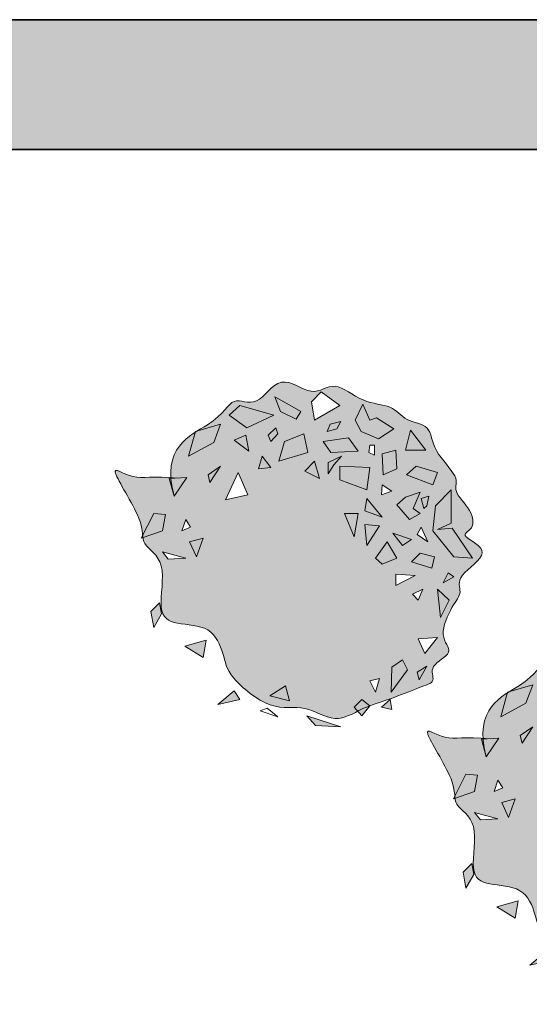
# Model space of a CAD drawing. Units: metres. Extents: x 4298.5 to 4325.2, y 2075 to 2095.8.
# Tile 13 of 35: x 4303.606 to 4304.508, y 2083.045 to 2084.788. Entities that reach past the tile are written whole.
import ezdxf

# ---------------------------------------------------------------- set-up
doc = ezdxf.new("R2010")
doc.units = ezdxf.units.M
for name, color, linetype, lineweight in [('A-ANNO-DIMS', 2, 'Continuous', 18), ('A-WALL', 7, 'Continuous', 35), ('A-WALL-PATT', 252, 'Continuous', 13), ('L-PLNT', 94, 'Continuous', 13)]:
    doc.layers.add(name, color=color, linetype=linetype, lineweight=lineweight)
doc.layers.add('L-PLNT-PATT', color=116, linetype='Continuous', lineweight=13, true_color=0x13823e)
doc.styles.get("Standard").update_dxf_attribs({"font": 'arial.ttf'})
doc.dimstyles.get("Standard").update_dxf_attribs({"dimtxt": 0.18, "dimasz": 0.18, "dimexe": 0.18, "dimexo": 0.0625, "dimgap": 0.09, "dimtad": 0, "dimtih": 1, "dimtoh": 1, "dimdec": 4, "dimzin": 0, "dimdsep": 46, "dimtxsty": 'Standard', "dimcen": 0.09, "dimadec": 0, "dimazin": 0, "dimtfac": 1, "dimtdec": 4, "dimtofl": 0, "dimtmove": 0, "dimatfit": 3, "dimfxl": 1, "dimtolj": 1, "dimtzin": 0, "dimarcsym": 0})

# ---------------------------------------------------------------- blocks, each defined once
blk = doc.blocks.new('*U9')
for points in [[(1.237, 12.003), (0.562, 11.31), (0.764, 10.013), (2.519, 11.051)], [(-4.432, 11.051), (-5.175, 10.359), (-3.96, 9.493), (-2.07, 10.359)], [(-2.003, 11.656), (-1.598, 10.618), (-0.518, 10.099), (-0.181, 10.618), (-0.788, 10.964)], [(4.139, 11.137), (3.599, 10.013), (4.004, 9.234), (5.218, 8.715), (6.298, 9.407), (5.083, 10.186), (4.611, 10.013)], [(-5.782, 9.753), (-7.537, 9.234), (-8.009, 7.504), (-6.255, 8.455)], [(2.586, 9.926), (1.844, 9.753), (1.642, 9.234), (2.316, 9.407)], [(-4.837, 8.628), (-3.825, 7.85), (-4.027, 8.974)], [(-1.935, 9.493), (-2.475, 8.974), (-2.273, 8.542), (-1.8, 9.061)], [(0.022, 9.061), (-1.328, 8.542), (-1.733, 7.157), (0.292, 7.763)], [(7.446, 9.32), (7.108, 7.936), (8.525, 7.936)], [(1.372, 8.542), (3.126, 8.801), (3.801, 7.85), (1.912, 7.763)], [(4.611, 8.282), (4.544, 7.763), (4.949, 7.59), (4.949, 8.282)], [(6.433, 7.936), (5.488, 7.676), (5.556, 6.206), (6.501, 6.638)], [(-2.88, 7.504), (-3.15, 6.638), (-2.273, 6.725)], [(0.764, 7.157), (0.089, 6.465), (1.102, 5.946)], [(1.709, 6.292), (1.709, 7.071), (2.654, 7.504), (2.114, 6.898)], [(-5.782, 6.811), (-6.659, 6.206), (-6.524, 5.687)], [(-4.567, 6.379), (-5.445, 4.475), (-3.892, 4.821)], [(2.519, 6.811), (2.519, 5.86), (4.409, 5.167), (4.611, 6.725)], [(7.851, 6.811), (7.176, 6.206), (8.998, 5.514), (9.335, 6.379)], [(-8.144, 6.033), (-9.359, 5.946), (-9.022, 4.735)], [(5.488, 5.514), (5.421, 4.821), (6.163, 5.081)], [(8.12, 4.994), (7.108, 4.648), (6.501, 4.129), (7.378, 3.091), (8.12, 3.524), (7.648, 3.87)], [(10.28, 5.167), (9.2, 4.043), (8.998, 2.312), (10.482, 0.495), (11.765, 0.409), (10.348, 2.485), (9.335, 2.399), (10.28, 2.831)], [(4.409, 4.562), (4.274, 3.697), (5.488, 3.264)], [(8.728, 4.735), (8.188, 4.562), (8.39, 3.87), (8.593, 4.043)], [(-11.316, 1.793), (-9.831, 2.312), (-9.629, 3.437), (-10.439, 3.524)], [(3.531, 1.88), (2.856, 3.524), (3.801, 3.524)], [(-8.212, 3.091), (-8.482, 2.312), (-7.874, 2.572)], [(4.274, 2.745), (5.286, 2.658), (4.409, 1.274)], [(7.513, 1.707), (6.906, 1.274), (6.231, 2.139)], [(8.188, 2.572), (7.918, 2.053), (8.66, 1.534)], [(-6.997, 1.793), (-7.942, 1.534), (-7.469, 0.495)], [(5.826, 1.534), (5.016, 0.409), (5.488, -0.024), (6.501, 0.409)], [(-8.212, 0.409), (-9.426, 0.322), (-9.831, 0.841)], [(8.12, 0.755), (7.513, 0.149), (8.93, -0.283), (9.133, 0.495)], [(10.078, -0.629), (9.74, -1.322), (10.482, -0.889)], [(7.783, -0.803), (6.433, -1.495), (6.433, -0.716)], [(8.323, -1.754), (7.985, -2.533), (7.581, -2.1)], [(9.335, -1.754), (9.538, -3.744), (10.145, -2.533)], [(-10.034, -2.706), (-10.641, -3.312), (-10.439, -4.436), (-9.899, -3.485)], [(-8.279, -5.734), (-6.794, -5.302), (-6.997, -6.513)], [(9.335, -5.129), (8.458, -6.253), (7.985, -5.215)], [(6.096, -8.935), (6.163, -7.205), (6.906, -6.686), (7.243, -7.378)], [(8.053, -8.07), (8.593, -7.118), (7.918, -7.551)], [(5.286, -7.984), (4.611, -8.157), (5.016, -8.935)], [(-4.837, -8.849), (-4.432, -9.454), (-5.985, -9.801)], [(-2.34, -9.195), (-1.26, -8.503), (-0.99, -9.541)], [(4.071, -9.454), (3.531, -9.974), (4.071, -10.579), (4.611, -9.887)], [(6.028, -9.454), (5.421, -9.974), (6.163, -10.147)], [(-2.543, -10.06), (-3.015, -10.233), (-1.8, -10.666)], [(0.224, -10.579), (0.832, -11.272), (2.586, -11.358)]]:
    blk.add_lwpolyline(points, close=True)
blk = doc.blocks.new('*D47')
at = {"layer": 'A-ANNO-DIMS', "color": 0, "lineweight": -2, "transparency": 16777216}
for p, q in [((4300.4306, 2084.4956), (4300.4306, 2074.9896)), ((4322.8106, 2084.4956), (4322.8106, 2074.9896)), ((4300.6106, 2075.1696), (4311.2252, 2075.1696)), ((4322.6306, 2075.1696), (4312.016, 2075.1696))]:
    blk.add_line(p, q, dxfattribs=at)
at = {"layer": 'A-ANNO-DIMS', "color": 0, "transparency": 16777216}
for points in [[(4300.6106, 2075.1996), (4300.6106, 2075.1396), (4300.4306, 2075.1696)], [(4322.6306, 2075.1996), (4322.6306, 2075.1396), (4322.8106, 2075.1696)]]:
    blk.add_solid(points, dxfattribs=at)
at = {"layer": 'Defpoints', "color": 0, "transparency": 16777216}
for p in [(4300.4306, 2084.5581), (4322.8106, 2084.5581), (4322.8106, 2075.1696)]:
    blk.add_point(p, dxfattribs=at)
at = {"layer": 'A-ANNO-DIMS', "color": 0, "transparency": 16777216, "insert": (4311.6206, 2075.1696), "char_height": 0.18, "attachment_point": 5}
blk.add_mtext('\\A1;22.38', dxfattribs=at)
blk = doc.blocks.new('*D51')
at = {"layer": 'A-ANNO-DIMS', "color": 0, "lineweight": -2, "transparency": 16777216}
for p, q in [((4305.5981, 2084.5581), (4299.0921, 2084.5581)), ((4299.2721, 2084.3781), (4299.2721, 2082.375)), ((4299.2721, 2080.0081), (4299.2721, 2082.0111)), ((4305.5981, 2079.8281), (4299.0921, 2079.8281))]:
    blk.add_line(p, q, dxfattribs=at)
at = {"layer": 'A-ANNO-DIMS', "color": 0, "transparency": 16777216}
for points in [[(4299.2421, 2084.3781), (4299.3021, 2084.3781), (4299.2721, 2084.5581)], [(4299.2421, 2080.0081), (4299.3021, 2080.0081), (4299.2721, 2079.8281)]]:
    blk.add_solid(points, dxfattribs=at)
at = {"layer": 'Defpoints', "color": 0, "transparency": 16777216}
for p in [(4305.6606, 2084.5581), (4299.2721, 2079.8281), (4305.6606, 2079.8281)]:
    blk.add_point(p, dxfattribs=at)
at = {"layer": 'A-ANNO-DIMS', "color": 0, "transparency": 16777216, "insert": (4299.2721, 2082.1931), "char_height": 0.18, "attachment_point": 5}
blk.add_mtext('\\A1;4.73', dxfattribs=at)
blk = doc.blocks.new('*D56')
at = {"layer": 'A-ANNO-DIMS', "color": 0, "lineweight": -2, "transparency": 16777216}
for p, q in [((4305.8281, 2085.0581), (4299.0921, 2085.0581)), ((4299.2721, 2084.8781), (4299.2721, 2083.74)), ((4299.2721, 2082.2381), (4299.2721, 2083.3761)), ((4305.8281, 2082.0581), (4299.0921, 2082.0581))]:
    blk.add_line(p, q, dxfattribs=at)
at = {"layer": 'A-ANNO-DIMS', "color": 0, "transparency": 16777216}
for points in [[(4299.2421, 2084.8781), (4299.3021, 2084.8781), (4299.2721, 2085.0581)], [(4299.2421, 2082.2381), (4299.3021, 2082.2381), (4299.2721, 2082.0581)]]:
    blk.add_solid(points, dxfattribs=at)
at = {"layer": 'Defpoints', "color": 0, "transparency": 16777216}
for p in [(4299.2721, 2085.0581), (4305.8906, 2085.0581), (4305.8906, 2082.0581)]:
    blk.add_point(p, dxfattribs=at)
at = {"layer": 'A-ANNO-DIMS', "color": 0, "transparency": 16777216, "insert": (4299.2721, 2083.5581), "char_height": 0.18, "attachment_point": 5}
blk.add_mtext('\\A1;3', dxfattribs=at)

msp = doc.modelspace()

# ---------------------------------------------------------------- hatches: boundary and pattern name
at = {"layer": 'A-WALL-PATT'}
h = msp.add_hatch(color=256, dxfattribs=at)
h.dxf.hatch_style = 1
h.paths.add_polyline_path([(4308.7606, 2094.4781), (4308.1606, 2094.4781), (4307.4606, 2094.4781), (4307.4606, 2094.2481), (4308.2706, 2094.2481), (4308.2706, 2094.1281), (4308.3906, 2094.1281), (4308.3906, 2094.2481), (4308.7606, 2094.2481)])
h.paths.add_polyline_path([(4310.1206, 2094.4781), (4309.5206, 2094.4781), (4309.5206, 2094.2481), (4309.8906, 2094.2481), (4309.8906, 2092.2481), (4308.3906, 2092.2481), (4308.3906, 2093.4281), (4308.2706, 2093.4281), (4308.2706, 2092.0181), (4309.8906, 2092.0181), (4309.8906, 2087.0181), (4309.7706, 2087.0181), (4309.7706, 2086.7881), (4309.8906, 2086.7881), (4311.9406, 2086.7881), (4311.9406, 2087.0181), (4310.1206, 2087.0181), (4310.1206, 2089.0181), (4310.2406, 2089.0181), (4310.2406, 2089.1381), (4310.1206, 2089.1381), (4310.1206, 2092.0181), (4310.3078, 2092.0181), (4310.3078, 2092.2481), (4310.1206, 2092.2481)])
h.paths.add_polyline_path([(4311.7406, 2092.2481), (4311.0678, 2092.2481), (4311.0678, 2092.0181), (4311.7406, 2092.0181)], flags=17)
h.paths.add_polyline_path([(4313.1733, 2092.2481), (4312.5006, 2092.2481), (4312.5006, 2092.0181), (4313.1733, 2092.0181)])
h.paths.add_polyline_path([(4314.5378, 2092.2481), (4314.1206, 2092.2481), (4313.9333, 2092.2481), (4313.9333, 2092.0181), (4314.1206, 2092.0181), (4314.1206, 2087.0181), (4314.0006, 2087.0181), (4314.0006, 2086.7881), (4314.1206, 2086.7881), (4315.5718, 2086.7881), (4315.5718, 2087.0181), (4314.3506, 2087.0181), (4314.3506, 2092.0181), (4314.5378, 2092.0181)])
h.paths.add_polyline_path([(4315.9706, 2092.2481), (4315.2978, 2092.2481), (4315.2978, 2092.0181), (4315.9706, 2092.0181)])
h.paths.add_polyline_path([(4317.4033, 2092.2481), (4316.7306, 2092.2481), (4316.7306, 2092.0181), (4317.4033, 2092.0181)])
h.paths.add_polyline_path([(4318.9506, 2092.2481), (4318.3506, 2092.2481), (4318.1633, 2092.2481), (4318.1633, 2092.0181), (4318.3506, 2092.0181), (4318.3506, 2091.8981), (4318.5806, 2091.8981), (4318.5806, 2092.0181), (4318.9506, 2092.0181)])
h.paths.add_polyline_path([(4321.0106, 2092.2481), (4319.7106, 2092.2481), (4319.7106, 2092.0181), (4320.0806, 2092.0181), (4320.0806, 2090.0181), (4318.5806, 2090.0181), (4318.5806, 2091.1981), (4318.3506, 2091.1981), (4318.3506, 2090.0181), (4318.3506, 2087.0181), (4318.2306, 2087.0181), (4318.2306, 2086.7881), (4318.3506, 2086.7881), (4318.3506, 2086.3081), (4318.5806, 2086.3081), (4318.5806, 2089.7881), (4321.7806, 2089.7881), (4321.7806, 2090.0181), (4320.2006, 2090.0181), (4320.2006, 2092.0181), (4321.0106, 2092.0181)])
h.paths.add_polyline_path([(4322.8106, 2092.2481), (4321.7706, 2092.2481), (4321.7706, 2092.0181), (4322.5806, 2092.0181), (4322.5806, 2091.2831), (4322.8106, 2091.2831)])
h.paths.add_polyline_path([(4322.8106, 2090.5231), (4322.5806, 2090.5231), (4322.5806, 2089.7881), (4322.5806, 2089.5254), (4322.8106, 2089.5254), (4322.8106, 2090.0181)])
h.paths.add_polyline_path([(4322.8106, 2088.7654), (4322.5806, 2088.7654), (4322.5806, 2087.6681), (4322.8106, 2087.6681)])
h.paths.add_polyline_path([(4322.8106, 2086.9081), (4322.5806, 2086.9081), (4322.5806, 2085.8107), (4322.8106, 2085.8107)])
h.paths.add_polyline_path([(4322.8106, 2085.0507), (4322.5806, 2085.0507), (4322.5806, 2084.7881), (4318.5806, 2084.7881), (4318.5806, 2085.0581), (4318.5806, 2085.4081), (4318.3506, 2085.4081), (4318.3506, 2084.5581), (4318.3506, 2080.8581), (4318.4706, 2080.8581), (4318.4706, 2082.3281), (4319.2606, 2082.3281), (4319.2606, 2082.5581), (4318.5806, 2082.5581), (4318.5806, 2084.5581), (4320.0806, 2084.5581), (4320.0806, 2083.9381), (4320.3106, 2083.9381), (4320.3106, 2084.5581), (4322.8106, 2084.5581)])
h.paths.add_polyline_path([(4320.3106, 2083.1781), (4320.0806, 2083.1781), (4320.0806, 2082.5581), (4319.9606, 2082.5581), (4319.9606, 2082.3281), (4320.0806, 2082.3281), (4320.0806, 2081.5731), (4320.3106, 2081.5731)], flags=17)
h.paths.add_polyline_path([(4320.3106, 2080.8131), (4320.0806, 2080.8131), (4320.0806, 2080.0581), (4318.4286, 2080.0581), (4318.4286, 2079.8281), (4320.3106, 2079.8281)])
h.paths.add_polyline_path([(4317.3506, 2085.2881), (4316.5718, 2085.2881), (4316.5718, 2085.0581), (4317.3506, 2085.0581)])
h.paths.add_polyline_path([(4315.5718, 2085.2881), (4314.8434, 2085.2881), (4314.8434, 2085.0581), (4315.5718, 2085.0581)])
h.paths.add_polyline_path([(4313.8434, 2085.2881), (4312.9406, 2085.2881), (4312.9406, 2085.0581), (4313.8434, 2085.0581)])
h.paths.add_polyline_path([(4311.9406, 2085.2881), (4311.4406, 2085.2881), (4311.4406, 2085.0581), (4311.9406, 2085.0581)])
h.paths.add_polyline_path([(4317.3306, 2087.0181), (4316.5718, 2087.0181), (4316.5718, 2086.7881), (4317.3306, 2086.7881)])
h.paths.add_polyline_path([(4313.1006, 2089.1381), (4311.1406, 2089.1381), (4311.1406, 2089.0181), (4312.9806, 2089.0181), (4312.9806, 2087.0181), (4312.9406, 2087.0181), (4312.9406, 2086.7881), (4313.1006, 2086.7881), (4313.1006, 2087.0181)])
h.paths.add_polyline_path([(4307.5515, 2087.0181), (4305.8906, 2087.0181), (4305.8906, 2092.2481), (4305.8906, 2094.2481), (4306.7006, 2094.2481), (4306.7006, 2094.4781), (4305.6606, 2094.4781), (4305.6606, 2092.2481), (4305.2906, 2092.2481), (4305.2906, 2092.0181), (4305.6606, 2092.0181), (4305.6606, 2090.0181), (4304.1606, 2090.0181), (4304.1606, 2091.1981), (4304.0406, 2091.1981), (4304.0406, 2089.9081), (4301.5606, 2089.9081), (4301.5606, 2089.7881), (4304.0406, 2089.7881), (4305.6606, 2089.7881), (4305.6606, 2086.6381), (4305.8906, 2086.6381), (4305.8906, 2086.7881), (4307.5515, 2086.7881)])
h.paths.add_polyline_path([(4307.5515, 2085.2881), (4305.8906, 2085.2881), (4305.8906, 2085.4381), (4305.6606, 2085.4381), (4305.6606, 2084.7881), (4305.2906, 2084.7881), (4305.2906, 2084.5581), (4305.6606, 2084.5581), (4305.6606, 2084.02), (4305.8906, 2084.02), (4305.8906, 2084.5581), (4305.8906, 2085.0581), (4307.5515, 2085.0581)])
h.paths.add_polyline_path([(4310.2406, 2085.2881), (4308.5515, 2085.2881), (4308.5515, 2085.0581), (4310.2406, 2085.0581)])
h.paths.add_polyline_path([(4317.4286, 2080.0581), (4316.5718, 2080.0581), (4316.5718, 2079.8281), (4317.4286, 2079.8281)])
h.paths.add_polyline_path([(4315.5718, 2080.0581), (4314.8434, 2080.0581), (4314.8434, 2079.8281), (4315.5718, 2079.8281)])
h.paths.add_polyline_path([(4313.8434, 2080.0581), (4312.9406, 2080.0581), (4312.9406, 2079.8281), (4313.8434, 2079.8281)])
h.paths.add_polyline_path([(4311.9406, 2080.0581), (4311.4406, 2080.0581), (4311.4406, 2079.8281), (4311.9406, 2079.8281)])
h.paths.add_polyline_path([(4310.2406, 2080.0581), (4310.1206, 2080.0581), (4310.1206, 2084.0381), (4309.8906, 2084.0381), (4309.8906, 2080.0581), (4309.1606, 2080.0581), (4309.1606, 2079.8281), (4310.2406, 2079.8281)])
h.paths.add_polyline_path([(4308.1606, 2080.0581), (4307.5106, 2080.0581), (4307.5106, 2080.1781), (4307.3906, 2080.1781), (4307.3906, 2080.0581), (4305.8906, 2080.0581), (4305.8906, 2080.567), (4305.6606, 2080.567), (4305.6606, 2079.8281), (4308.1606, 2079.8281)])
h.paths.add_polyline_path([(4307.5106, 2081.9381), (4309.0906, 2081.9381), (4309.0906, 2082.0581), (4305.8906, 2082.0581), (4305.8906, 2083.26), (4305.6606, 2083.26), (4305.6606, 2081.327), (4305.8906, 2081.327), (4305.8906, 2081.9381), (4307.3906, 2081.9381), (4307.3906, 2080.8781), (4307.5106, 2080.8781)])
h.paths.add_polyline_path([(4304.5306, 2084.7881), (4302.7306, 2084.7881), (4302.7306, 2084.5581), (4304.5306, 2084.5581)])
h.paths.add_polyline_path([(4301.9706, 2084.7881), (4300.6606, 2084.7881), (4300.6606, 2085.0249), (4300.4306, 2085.0249), (4300.4306, 2084.5581), (4301.9706, 2084.5581)])
h.paths.add_polyline_path([(4300.6606, 2086.8843), (4300.4306, 2086.8843), (4300.4306, 2085.7849), (4300.6606, 2085.7849)])
h.paths.add_polyline_path([(4300.6606, 2089.1618), (4300.4306, 2089.1618), (4300.4306, 2087.6443), (4300.6606, 2087.6443)])
h.paths.add_polyline_path([(4300.6606, 2091.0212), (4300.4306, 2091.0212), (4300.4306, 2089.9218), (4300.6606, 2089.9218)])
h.paths.add_polyline_path([(4300.6606, 2092.0181), (4301.9706, 2092.0181), (4301.9706, 2092.2481), (4300.4306, 2092.2481), (4300.4306, 2091.7812), (4300.6606, 2091.7812)])
h.paths.add_polyline_path([(4304.5306, 2092.2481), (4302.7306, 2092.2481), (4302.7306, 2092.0181), (4304.0406, 2092.0181), (4304.0406, 2091.8981), (4304.1606, 2091.8981), (4304.1606, 2092.0181), (4304.5306, 2092.0181)], flags=17)
at = {"layer": 'L-PLNT-PATT'}
h = msp.add_hatch(color=256, dxfattribs=at)
h.dxf.hatch_style = 1
edge = h.paths.add_edge_path()
edge.add_spline(control_points=[(4304.2042, 2083.5639), (4304.2068, 2083.5652), (4304.2254, 2083.5745), (4304.2612, 2083.5843), (4304.3157, 2083.6076), (4304.3451, 2083.6152), (4304.3264, 2083.6436), (4304.3789, 2083.6678), (4304.3452, 2083.6942), (4304.3722, 2083.7539), (4304.391, 2083.7734), (4304.3743, 2083.8019), (4304.4485, 2083.8467), (4304.3786, 2083.8763), (4304.4113, 2083.8839), (4304.4073, 2083.9191), (4304.3692, 2083.9557), (4304.3878, 2083.975), (4304.3347, 2084.026), (4304.3347, 2084.0721), (4304.2869, 2084.0754), (4304.2664, 2084.1073), (4304.2132, 2084.1073), (4304.1609, 2084.1527), (4304.1261, 2084.1156), (4304.0654, 2084.1664), (4304.0255, 2084.0964), (4303.981, 2084.1263), (4303.9666, 2084.0869), (4303.9263, 2084.0639), (4303.92, 2084.06)], knot_values=[0.818571, 0.818571, 0.818571, 0.818571, 0.97924, 1.97924, 2.97924, 3.97924, 4.97924, 5.97924, 6.97924, 7.97924, 8.97924, 9.97924, 10.97924, 11.97924, 12.97924, 13.97924, 14.97924, 15.97924, 16.97924, 17.97924, 18.97924, 19.97924, 20.97924, 21.97924, 22.97924, 23.97924, 24.97924, 25.97924, 26.97924, 27.16067, 27.16067, 27.16067, 27.16067], degree=3, periodic=0)
edge.add_line((4303.92, 2084.06), (4303.9612, 2084.0722))
edge.add_line((4303.9612, 2084.0722), (4303.9492, 2084.0392))
edge.add_line((4303.9492, 2084.0392), (4303.9047, 2084.015))
edge.add_line((4303.9047, 2084.015), (4303.9163, 2084.0576))
edge.add_spline(control_points=[(4303.9163, 2084.0576), (4303.8936, 2084.043), (4303.8703, 2084.022), (4303.8731, 2083.9776)], knot_values=[0.141368, 0.141368, 0.141368, 0.141368, 0.783694, 0.783694, 0.783694, 0.783694], degree=3, periodic=0)
edge.add_spline(control_points=[(4303.8731, 2083.9776), (4303.877, 2083.9774), (4303.8813, 2083.977), (4303.8858, 2083.9766)], knot_values=[40.901028, 40.901028, 40.901028, 40.901028, 41, 41, 41, 41], degree=3, periodic=0)
edge.add_line((4303.8858, 2083.9766), (4303.9012, 2083.9777))
edge.add_line((4303.9012, 2083.9777), (4303.8789, 2083.9447))
edge.add_line((4303.8789, 2083.9447), (4303.8704, 2083.9755))
edge.add_line((4303.8704, 2083.9755), (4303.8732, 2083.9757))
edge.add_spline(control_points=[(4303.8732, 2083.9757), (4303.8732, 2083.9763), (4303.8731, 2083.977), (4303.8731, 2083.9776)], knot_values=[0.13204, 0.13204, 0.13204, 0.13204, 0.141368, 0.141368, 0.141368, 0.141368], degree=3, periodic=0)
edge.add_spline(control_points=[(4303.8731, 2083.9776), (4303.8369, 2083.98), (4303.8052, 2083.9701), (4303.7532, 2084.0121), (4303.8203, 2083.9096), (4303.8226, 2083.8827), (4303.8233, 2083.8752)], knot_values=[37.439141, 37.439141, 37.439141, 37.439141, 38.340169, 39.340169, 40.340169, 40.901028, 40.901028, 40.901028, 40.901028], degree=3, periodic=0)
edge.add_line((4303.8233, 2083.8752), (4303.8429, 2083.914))
edge.add_line((4303.8429, 2083.914), (4303.8635, 2083.9117))
edge.add_line((4303.8635, 2083.9117), (4303.8584, 2083.8832))
edge.add_line((4303.8584, 2083.8832), (4303.8237, 2083.8711))
edge.add_spline(control_points=[(4303.8237, 2083.8711), (4303.8242, 2083.8671), (4303.8273, 2083.8536), (4303.8687, 2083.8326), (4303.8472, 2083.7353), (4303.8795, 2083.7165), (4303.9457, 2083.7165), (4303.9684, 2083.6628), (4303.9719, 2083.6273), (4304.0529, 2083.5612), (4304.1112, 2083.578), (4304.1616, 2083.5411), (4304.1908, 2083.5571), (4304.2042, 2083.5639)], knot_values=[27.16067, 27.16067, 27.16067, 27.16067, 27.490087, 28.490087, 29.490087, 30.490087, 31.490087, 32.490087, 33.490087, 34.490087, 35.490087, 36.490087, 37.329418, 37.329418, 37.329418, 37.329418], degree=3, periodic=0)
edge.add_line((4304.2042, 2083.5639), (4304.1978, 2083.5711))
edge.add_line((4304.1978, 2083.5711), (4304.2115, 2083.5843))
edge.add_line((4304.2115, 2083.5843), (4304.2252, 2083.5733))
h.paths.add_polyline_path([(4304.1806, 2083.914), (4304.2046, 2083.914), (4304.1978, 2083.8722)], flags=16)
h.paths.add_polyline_path([(4304.2166, 2083.8942), (4304.2424, 2083.892), (4304.2201, 2083.8568)], flags=16)
h.paths.add_polyline_path([(4304.0092, 2083.9469), (4303.9698, 2083.9381), (4303.9921, 2083.9865)], flags=16)
h.paths.add_polyline_path([(4304.1361, 2083.9755), (4304.1103, 2083.9887), (4304.1275, 2084.0062)], flags=16)
h.paths.add_polyline_path([(4304.2166, 2083.9183), (4304.2201, 2083.9403), (4304.2475, 2083.9074)], flags=16)
h.paths.add_polyline_path([(4304.2355, 2083.8348), (4304.2561, 2083.8634), (4304.2732, 2083.8348), (4304.2475, 2083.8238)], flags=16)
h.paths.add_polyline_path([(4304.1721, 2083.9733), (4304.1721, 2083.9974), (4304.2252, 2083.9953), (4304.2201, 2083.9557)], flags=16)
h.paths.add_polyline_path([(4304.1515, 2083.9843), (4304.1515, 2084.004), (4304.1755, 2084.015), (4304.1618, 2083.9997)], flags=16)
h.paths.add_polyline_path([(4304.0504, 2083.9953), (4304.0281, 2083.9931), (4304.0349, 2084.015)], flags=16)
h.paths.add_polyline_path([(4304.0641, 2084.0062), (4304.0744, 2084.0414), (4304.1086, 2084.0546), (4304.1155, 2084.0216)], flags=16)
h.paths.add_polyline_path([(4303.9304, 2083.87), (4303.9184, 2083.837), (4303.9064, 2083.8634)], flags=16)
h.paths.add_polyline_path([(4304.2664, 2083.8788), (4304.2989, 2083.8678), (4304.2835, 2083.8568)], flags=16)
h.paths.add_polyline_path([(4304.2458, 2083.9469), (4304.2475, 2083.9645), (4304.2646, 2083.9535)], flags=16)
h.paths.add_polyline_path([(4304.1567, 2084.0216), (4304.1429, 2084.0414), (4304.1875, 2084.048), (4304.2046, 2084.0238)], flags=16)
h.paths.add_polyline_path([(4304.2715, 2083.8063), (4304.3058, 2083.804), (4304.2715, 2083.7865)], flags=16)
h.paths.add_polyline_path([(4303.9081, 2083.8898), (4303.8926, 2083.8832), (4303.8995, 2083.903)], flags=16)
h.paths.add_polyline_path([(4304.0109, 2084.0238), (4303.9852, 2084.0436), (4304.0058, 2084.0524)], flags=16)
h.paths.add_polyline_path([(4303.9424, 2083.9689), (4303.939, 2083.9821), (4303.9612, 2083.9974)], flags=16)
h.paths.add_polyline_path([(4304.0504, 2084.0414), (4304.0452, 2084.0524), (4304.0589, 2084.0656), (4304.0624, 2084.0546)], flags=16)
h.paths.add_polyline_path([(4304.2732, 2083.9293), (4304.2886, 2083.9425), (4304.3143, 2083.9513), (4304.3023, 2083.9227), (4304.3143, 2083.914), (4304.2955, 2083.903)], flags=16)
h.paths.add_polyline_path([(4303.8995, 2083.8348), (4303.8687, 2083.8326), (4303.8584, 2083.8458)], flags=16)
h.paths.add_polyline_path([(4304.2492, 2083.9821), (4304.2475, 2084.0194), (4304.2715, 2084.026), (4304.2732, 2083.9931)], flags=16)
h.paths.add_polyline_path([(4304.2989, 2083.8282), (4304.3143, 2083.8436), (4304.3401, 2083.837), (4304.3349, 2083.8173)], flags=16)
h.paths.add_polyline_path([(4304.2235, 2084.0216), (4304.2252, 2084.0348), (4304.2338, 2084.0348), (4304.2338, 2084.0172)], flags=16)
h.paths.add_polyline_path([(4304.1498, 2084.059), (4304.1549, 2084.0722), (4304.1738, 2084.0766), (4304.1669, 2084.0634)], flags=16)
h.paths.add_polyline_path([(4304.3092, 2083.8766), (4304.3161, 2083.8898), (4304.3281, 2083.8634)], flags=16)
h.paths.add_polyline_path([(4304.3006, 2083.7711), (4304.3195, 2083.7799), (4304.3109, 2083.7601)], flags=16)
h.paths.add_polyline_path([(4304.0949, 2084.081), (4304.0675, 2084.0941), (4304.0572, 2084.1205), (4304.0881, 2084.1029), (4304.1035, 2084.0941)], flags=16)
h.paths.add_polyline_path([(4304.1275, 2084.0788), (4304.1224, 2084.1117), (4304.1395, 2084.1293), (4304.1721, 2084.1051)], flags=16)
h.paths.add_polyline_path([(4304.0075, 2084.0656), (4303.9766, 2084.0876), (4303.9955, 2084.1051), (4304.0555, 2084.0876)], flags=16)
h.paths.add_polyline_path([(4304.2904, 2083.9821), (4304.3075, 2083.9974), (4304.3452, 2083.9865), (4304.3366, 2083.9645)], flags=16)
h.paths.add_polyline_path([(4304.2098, 2084.059), (4304.1995, 2084.0788), (4304.2132, 2084.1073), (4304.2252, 2084.0788), (4304.2372, 2084.0832), (4304.2681, 2084.0634), (4304.2406, 2084.0458)], flags=16)
h.paths.add_polyline_path([(4304.3212, 2083.9227), (4304.3161, 2083.9403), (4304.3298, 2083.9447), (4304.3264, 2083.9271)], flags=16)
h.paths.add_polyline_path([(4304.3366, 2083.8832), (4304.3418, 2083.9271), (4304.3692, 2083.9557), (4304.3692, 2083.8964), (4304.3452, 2083.8854), (4304.3709, 2083.8876), (4304.4069, 2083.8348), (4304.3743, 2083.837)], flags=16)
h.paths.add_polyline_path([(4304.0761, 2083.6085), (4304.0829, 2083.5821), (4304.0487, 2083.5909)], flags=16)
h.paths.add_polyline_path([(4304.2886, 2084.026), (4304.2972, 2084.0612), (4304.3246, 2084.026)], flags=16)
h.paths.add_polyline_path([(4304.3452, 2083.7799), (4304.3658, 2083.7601), (4304.3504, 2083.7293)], flags=16)
h.paths.add_polyline_path([(4304.3555, 2083.7909), (4304.3641, 2083.8085), (4304.3743, 2083.8019)], flags=16)
h.paths.add_polyline_path([(4304.2252, 2083.6173), (4304.2424, 2083.6217), (4304.2355, 2083.5975)], flags=16)
h.paths.add_polyline_path([(4304.3109, 2083.692), (4304.3452, 2083.6942), (4304.3229, 2083.6656)], flags=16)
h.paths.add_polyline_path([(4304.2646, 2083.6414), (4304.2835, 2083.6546), (4304.2921, 2083.637), (4304.2629, 2083.5975)], flags=16)
h.paths.add_polyline_path([(4304.3092, 2083.6326), (4304.3264, 2083.6436), (4304.3126, 2083.6195)], flags=16)
h = msp.add_hatch(color=256, dxfattribs=at)
h.dxf.hatch_style = 1
h.paths.add_polyline_path([(4304.2201, 2083.9557), (4304.2252, 2083.9953), (4304.1721, 2083.9974), (4304.1721, 2083.9733)])
h.paths.add_polyline_path([(4304.2664, 2083.8788), (4304.2835, 2083.8568), (4304.2989, 2083.8678)])
h.paths.add_polyline_path([(4304.2475, 2084.0194), (4304.2492, 2083.9821), (4304.2732, 2083.9931), (4304.2715, 2084.026)])
h.paths.add_polyline_path([(4304.2681, 2084.0634), (4304.2372, 2084.0832), (4304.2252, 2084.0788), (4304.2132, 2084.1073), (4304.1995, 2084.0788), (4304.2098, 2084.059), (4304.2406, 2084.0458)])
h.paths.add_polyline_path([(4304.1138, 2083.5557), (4304.1292, 2083.5381), (4304.1738, 2083.536)])
h.paths.add_polyline_path([(4304.0949, 2084.081), (4304.1035, 2084.0941), (4304.0881, 2084.1029), (4304.0572, 2084.1205), (4304.0675, 2084.0941)])
h.paths.add_polyline_path([(4303.9955, 2084.1051), (4303.9766, 2084.0876), (4304.0075, 2084.0656), (4304.0555, 2084.0876)])
h.paths.add_polyline_path([(4304.0744, 2084.0414), (4304.0641, 2084.0062), (4304.1155, 2084.0216), (4304.1086, 2084.0546)])
h.paths.add_polyline_path([(4304.0624, 2084.0546), (4304.0589, 2084.0656), (4304.0452, 2084.0524), (4304.0504, 2084.0414)])
h.paths.add_polyline_path([(4304.0349, 2084.015), (4304.0281, 2083.9931), (4304.0504, 2083.9953)])
h.paths.add_polyline_path([(4304.0109, 2084.0238), (4304.0058, 2084.0524), (4303.9852, 2084.0436)])
h.paths.add_polyline_path([(4303.9166, 2084.059), (4303.9047, 2084.015), (4303.9492, 2084.0392), (4303.9612, 2084.0722)])
h.paths.add_polyline_path([(4303.9612, 2083.9974), (4303.939, 2083.9821), (4303.9424, 2083.9689)])
h.paths.add_polyline_path([(4303.8704, 2083.9755), (4303.8789, 2083.9447), (4303.9012, 2083.9777)])
h.paths.add_polyline_path([(4303.8207, 2083.87), (4303.8584, 2083.8832), (4303.8635, 2083.9117), (4303.8429, 2083.914)])
h.paths.add_polyline_path([(4303.9304, 2083.87), (4303.9064, 2083.8634), (4303.9184, 2083.837)])
h.paths.add_polyline_path([(4303.8567, 2083.7359), (4303.8532, 2083.7557), (4303.8378, 2083.7403), (4303.8429, 2083.7118)])
h.paths.add_polyline_path([(4303.9355, 2083.6898), (4303.8978, 2083.6788), (4303.9304, 2083.659)])
h.paths.add_polyline_path([(4303.9561, 2083.5755), (4303.9955, 2083.5843), (4303.9852, 2083.5997)])
h.paths.add_polyline_path([(4304.0761, 2083.6085), (4304.0487, 2083.5909), (4304.0829, 2083.5821)])
h.paths.add_polyline_path([(4304.2115, 2083.5843), (4304.1978, 2083.5711), (4304.2115, 2083.5557), (4304.2252, 2083.5733)])
h.paths.add_polyline_path([(4304.2921, 2083.637), (4304.2835, 2083.6546), (4304.2646, 2083.6414), (4304.2629, 2083.5975)])
h.paths.add_polyline_path([(4304.2612, 2083.5843), (4304.2458, 2083.5711), (4304.2646, 2083.5667)])
h.paths.add_polyline_path([(4304.3092, 2083.6326), (4304.3126, 2083.6195), (4304.3264, 2083.6436)])
h.paths.add_polyline_path([(4304.3504, 2083.7293), (4304.3658, 2083.7601), (4304.3452, 2083.7799)])
h.paths.add_polyline_path([(4304.2355, 2083.8348), (4304.2475, 2083.8238), (4304.2732, 2083.8348), (4304.2561, 2083.8634)])
h.paths.add_polyline_path([(4304.3743, 2083.837), (4304.4069, 2083.8348), (4304.3709, 2083.8876), (4304.3452, 2083.8854), (4304.3692, 2083.8964), (4304.3692, 2083.9557), (4304.3418, 2083.9271), (4304.3366, 2083.8832)])
h.paths.add_polyline_path([(4304.3143, 2083.8436), (4304.2989, 2083.8282), (4304.3349, 2083.8173), (4304.3401, 2083.837)])
h.paths.add_polyline_path([(4304.3743, 2083.8019), (4304.3641, 2083.8085), (4304.3555, 2083.7909)])
h.paths.add_polyline_path([(4304.3143, 2083.9513), (4304.2886, 2083.9425), (4304.2732, 2083.9293), (4304.2955, 2083.903), (4304.3143, 2083.914), (4304.3023, 2083.9227)])
h.paths.add_polyline_path([(4304.3161, 2083.9403), (4304.3212, 2083.9227), (4304.3264, 2083.9271), (4304.3298, 2083.9447)])
h.paths.add_polyline_path([(4304.3366, 2083.9645), (4304.3452, 2083.9865), (4304.3075, 2083.9974), (4304.2904, 2083.9821)])
h.paths.add_polyline_path([(4304.2475, 2083.9074), (4304.2201, 2083.9403), (4304.2166, 2083.9183)])
h.paths.add_polyline_path([(4304.2046, 2083.914), (4304.1806, 2083.914), (4304.1978, 2083.8722)])
h.paths.add_polyline_path([(4304.2424, 2083.892), (4304.2166, 2083.8942), (4304.2201, 2083.8568)])
h.paths.add_polyline_path([(4304.2046, 2084.0238), (4304.1875, 2084.048), (4304.1429, 2084.0414), (4304.1567, 2084.0216)])
h.paths.add_polyline_path([(4304.1618, 2083.9997), (4304.1755, 2084.015), (4304.1515, 2084.004), (4304.1515, 2083.9843)])
h.paths.add_polyline_path([(4304.1275, 2084.0062), (4304.1103, 2083.9887), (4304.1361, 2083.9755)])
h.paths.add_polyline_path([(4304.1669, 2084.0634), (4304.1738, 2084.0766), (4304.1549, 2084.0722), (4304.1498, 2084.059)])
h.paths.add_polyline_path([(4304.2972, 2084.0612), (4304.2886, 2084.026), (4304.3246, 2084.026)])
h = msp.add_hatch(color=256, dxfattribs=at)
h.dxf.hatch_style = 1
edge = h.paths.add_edge_path()
edge.add_spline(control_points=[(4304.7568, 2083.1024), (4304.7594, 2083.1037), (4304.778, 2083.1131), (4304.8138, 2083.1228), (4304.8683, 2083.1461), (4304.8977, 2083.1537), (4304.8789, 2083.1822), (4304.9315, 2083.2063), (4304.8978, 2083.2327), (4304.9248, 2083.2924), (4304.9435, 2083.3119), (4304.9269, 2083.3404), (4305.0011, 2083.3852), (4304.9312, 2083.4148), (4304.9639, 2083.4224), (4304.9599, 2083.4576), (4304.9218, 2083.4942), (4304.9404, 2083.5135), (4304.8873, 2083.5645), (4304.8873, 2083.6106), (4304.8395, 2083.6139), (4304.819, 2083.6458), (4304.7658, 2083.6458), (4304.7135, 2083.6912), (4304.6787, 2083.6541), (4304.618, 2083.7049), (4304.5781, 2083.6349), (4304.5335, 2083.6648), (4304.5192, 2083.6255), (4304.4789, 2083.6024), (4304.4725, 2083.5985)], knot_values=[0.818571, 0.818571, 0.818571, 0.818571, 0.97924, 1.97924, 2.97924, 3.97924, 4.97924, 5.97924, 6.97924, 7.97924, 8.97924, 9.97924, 10.97924, 11.97924, 12.97924, 13.97924, 14.97924, 15.97924, 16.97924, 17.97924, 18.97924, 19.97924, 20.97924, 21.97924, 22.97924, 23.97924, 24.97924, 25.97924, 26.97924, 27.16067, 27.16067, 27.16067, 27.16067], degree=3, periodic=0)
edge.add_line((4304.4725, 2083.5985), (4304.5138, 2083.6107))
edge.add_line((4304.5138, 2083.6107), (4304.5018, 2083.5777))
edge.add_line((4304.5018, 2083.5777), (4304.4572, 2083.5536))
edge.add_line((4304.4572, 2083.5536), (4304.4689, 2083.5961))
edge.add_spline(control_points=[(4304.4689, 2083.5961), (4304.4462, 2083.5815), (4304.4229, 2083.5605), (4304.4256, 2083.5161)], knot_values=[0.141368, 0.141368, 0.141368, 0.141368, 0.783694, 0.783694, 0.783694, 0.783694], degree=3, periodic=0)
edge.add_spline(control_points=[(4304.4256, 2083.5161), (4304.4296, 2083.5159), (4304.4339, 2083.5155), (4304.4384, 2083.5151)], knot_values=[40.901028, 40.901028, 40.901028, 40.901028, 41, 41, 41, 41], degree=3, periodic=0)
edge.add_line((4304.4384, 2083.5151), (4304.4538, 2083.5162))
edge.add_line((4304.4538, 2083.5162), (4304.4315, 2083.4832))
edge.add_line((4304.4315, 2083.4832), (4304.423, 2083.514))
edge.add_line((4304.423, 2083.514), (4304.4258, 2083.5142))
edge.add_spline(control_points=[(4304.4258, 2083.5142), (4304.4257, 2083.5148), (4304.4257, 2083.5155), (4304.4256, 2083.5161)], knot_values=[0.13204, 0.13204, 0.13204, 0.13204, 0.141368, 0.141368, 0.141368, 0.141368], degree=3, periodic=0)
edge.add_spline(control_points=[(4304.4256, 2083.5161), (4304.3894, 2083.5185), (4304.3578, 2083.5086), (4304.3058, 2083.5506), (4304.3729, 2083.4481), (4304.3752, 2083.4212), (4304.3759, 2083.4137)], knot_values=[37.439141, 37.439141, 37.439141, 37.439141, 38.340169, 39.340169, 40.340169, 40.901028, 40.901028, 40.901028, 40.901028], degree=3, periodic=0)
edge.add_line((4304.3759, 2083.4137), (4304.3955, 2083.4525))
edge.add_line((4304.3955, 2083.4525), (4304.4161, 2083.4502))
edge.add_line((4304.4161, 2083.4502), (4304.411, 2083.4217))
edge.add_line((4304.411, 2083.4217), (4304.3763, 2083.4096))
edge.add_spline(control_points=[(4304.3763, 2083.4096), (4304.3768, 2083.4056), (4304.3799, 2083.3921), (4304.4212, 2083.3711), (4304.3998, 2083.2738), (4304.432, 2083.255), (4304.4983, 2083.255), (4304.521, 2083.2013), (4304.5245, 2083.1658), (4304.6055, 2083.0997), (4304.6638, 2083.1165), (4304.7142, 2083.0796), (4304.7433, 2083.0956), (4304.7568, 2083.1024)], knot_values=[27.16067, 27.16067, 27.16067, 27.16067, 27.490087, 28.490087, 29.490087, 30.490087, 31.490087, 32.490087, 33.490087, 34.490087, 35.490087, 36.490087, 37.329418, 37.329418, 37.329418, 37.329418], degree=3, periodic=0)
edge.add_line((4304.7568, 2083.1024), (4304.7504, 2083.1096))
edge.add_line((4304.7504, 2083.1096), (4304.7641, 2083.1228))
edge.add_line((4304.7641, 2083.1228), (4304.7778, 2083.1118))
h.paths.add_polyline_path([(4304.7332, 2083.4525), (4304.7572, 2083.4525), (4304.7504, 2083.4107)], flags=16)
h.paths.add_polyline_path([(4304.7692, 2083.4327), (4304.7949, 2083.4305), (4304.7727, 2083.3953)], flags=16)
h.paths.add_polyline_path([(4304.5618, 2083.4854), (4304.5224, 2083.4766), (4304.5447, 2083.525)], flags=16)
h.paths.add_polyline_path([(4304.6887, 2083.514), (4304.6629, 2083.5272), (4304.6801, 2083.5447)], flags=16)
h.paths.add_polyline_path([(4304.7692, 2083.4569), (4304.7727, 2083.4788), (4304.8001, 2083.4459)], flags=16)
h.paths.add_polyline_path([(4304.7881, 2083.3733), (4304.8087, 2083.4019), (4304.8258, 2083.3733), (4304.8001, 2083.3623)], flags=16)
h.paths.add_polyline_path([(4304.7247, 2083.5118), (4304.7247, 2083.5359), (4304.7778, 2083.5338), (4304.7727, 2083.4942)], flags=16)
h.paths.add_polyline_path([(4304.7041, 2083.5228), (4304.7041, 2083.5426), (4304.7281, 2083.5536), (4304.7144, 2083.5382)], flags=16)
h.paths.add_polyline_path([(4304.6029, 2083.5338), (4304.5807, 2083.5316), (4304.5875, 2083.5536)], flags=16)
h.paths.add_polyline_path([(4304.6167, 2083.5447), (4304.6269, 2083.5799), (4304.6612, 2083.5931), (4304.6681, 2083.5601)], flags=16)
h.paths.add_polyline_path([(4304.4829, 2083.4085), (4304.471, 2083.3755), (4304.4589, 2083.4019)], flags=16)
h.paths.add_polyline_path([(4304.8189, 2083.4173), (4304.8515, 2083.4063), (4304.8361, 2083.3953)], flags=16)
h.paths.add_polyline_path([(4304.7984, 2083.4854), (4304.8001, 2083.503), (4304.8172, 2083.492)], flags=16)
h.paths.add_polyline_path([(4304.7092, 2083.5601), (4304.6955, 2083.5799), (4304.7401, 2083.5865), (4304.7572, 2083.5623)], flags=16)
h.paths.add_polyline_path([(4304.8241, 2083.3448), (4304.8584, 2083.3426), (4304.8241, 2083.325)], flags=16)
h.paths.add_polyline_path([(4304.4607, 2083.4283), (4304.4452, 2083.4217), (4304.4521, 2083.4415)], flags=16)
h.paths.add_polyline_path([(4304.5635, 2083.5623), (4304.5378, 2083.5821), (4304.5584, 2083.5909)], flags=16)
h.paths.add_polyline_path([(4304.495, 2083.5074), (4304.4915, 2083.5206), (4304.5138, 2083.5359)], flags=16)
h.paths.add_polyline_path([(4304.6029, 2083.5799), (4304.5978, 2083.5909), (4304.6115, 2083.6041), (4304.615, 2083.5931)], flags=16)
h.paths.add_polyline_path([(4304.8258, 2083.4678), (4304.8412, 2083.481), (4304.8669, 2083.4898), (4304.8549, 2083.4612), (4304.8669, 2083.4525), (4304.8481, 2083.4415)], flags=16)
h.paths.add_polyline_path([(4304.4521, 2083.3733), (4304.4212, 2083.3711), (4304.411, 2083.3843)], flags=16)
h.paths.add_polyline_path([(4304.8018, 2083.5206), (4304.8001, 2083.5579), (4304.8241, 2083.5645), (4304.8258, 2083.5316)], flags=16)
h.paths.add_polyline_path([(4304.8515, 2083.3667), (4304.8669, 2083.3821), (4304.8926, 2083.3755), (4304.8875, 2083.3558)], flags=16)
h.paths.add_polyline_path([(4304.7761, 2083.5601), (4304.7778, 2083.5733), (4304.7864, 2083.5733), (4304.7864, 2083.5557)], flags=16)
h.paths.add_polyline_path([(4304.7024, 2083.5975), (4304.7075, 2083.6107), (4304.7264, 2083.6151), (4304.7195, 2083.6019)], flags=16)
h.paths.add_polyline_path([(4304.8618, 2083.4151), (4304.8686, 2083.4283), (4304.8806, 2083.4019)], flags=16)
h.paths.add_polyline_path([(4304.8532, 2083.3096), (4304.8721, 2083.3184), (4304.8635, 2083.2986)], flags=16)
h.paths.add_polyline_path([(4304.6475, 2083.6195), (4304.6201, 2083.6326), (4304.6098, 2083.659), (4304.6407, 2083.6414), (4304.6561, 2083.6326)], flags=16)
h.paths.add_polyline_path([(4304.6801, 2083.6173), (4304.6749, 2083.6502), (4304.6921, 2083.6678), (4304.7247, 2083.6436)], flags=16)
h.paths.add_polyline_path([(4304.5601, 2083.6041), (4304.5292, 2083.6261), (4304.5481, 2083.6436), (4304.6081, 2083.6261)], flags=16)
h.paths.add_polyline_path([(4304.8429, 2083.5206), (4304.8601, 2083.5359), (4304.8978, 2083.525), (4304.8892, 2083.503)], flags=16)
h.paths.add_polyline_path([(4304.7624, 2083.5975), (4304.7521, 2083.6173), (4304.7658, 2083.6458), (4304.7778, 2083.6173), (4304.7898, 2083.6217), (4304.8206, 2083.6019), (4304.7932, 2083.5843)], flags=16)
h.paths.add_polyline_path([(4304.8738, 2083.4612), (4304.8686, 2083.4788), (4304.8824, 2083.4832), (4304.8789, 2083.4656)], flags=16)
h.paths.add_polyline_path([(4304.8892, 2083.4217), (4304.8944, 2083.4656), (4304.9218, 2083.4942), (4304.9218, 2083.4349), (4304.8978, 2083.4239), (4304.9235, 2083.4261), (4304.9595, 2083.3733), (4304.9269, 2083.3755)], flags=16)
h.paths.add_polyline_path([(4304.6287, 2083.147), (4304.6355, 2083.1206), (4304.6012, 2083.1294)], flags=16)
h.paths.add_polyline_path([(4304.8412, 2083.5645), (4304.8498, 2083.5997), (4304.8772, 2083.5645)], flags=16)
h.paths.add_polyline_path([(4304.8978, 2083.3184), (4304.9184, 2083.2986), (4304.9029, 2083.2679)], flags=16)
h.paths.add_polyline_path([(4304.9081, 2083.3294), (4304.9167, 2083.347), (4304.9269, 2083.3404)], flags=16)
h.paths.add_polyline_path([(4304.7778, 2083.1558), (4304.7949, 2083.1602), (4304.7881, 2083.136)], flags=16)
h.paths.add_polyline_path([(4304.8635, 2083.2305), (4304.8978, 2083.2327), (4304.8755, 2083.2041)], flags=16)
h.paths.add_polyline_path([(4304.8172, 2083.1799), (4304.8361, 2083.1931), (4304.8446, 2083.1755), (4304.8155, 2083.136)], flags=16)
h.paths.add_polyline_path([(4304.8618, 2083.1712), (4304.8789, 2083.1822), (4304.8652, 2083.158)], flags=16)
h = msp.add_hatch(color=256, dxfattribs=at)
h.dxf.hatch_style = 1
h.paths.add_polyline_path([(4304.7727, 2083.4942), (4304.7778, 2083.5338), (4304.7247, 2083.5359), (4304.7247, 2083.5118)])
h.paths.add_polyline_path([(4304.8189, 2083.4173), (4304.8361, 2083.3953), (4304.8515, 2083.4063)])
h.paths.add_polyline_path([(4304.8001, 2083.5579), (4304.8018, 2083.5206), (4304.8258, 2083.5316), (4304.8241, 2083.5645)])
h.paths.add_polyline_path([(4304.8206, 2083.6019), (4304.7898, 2083.6217), (4304.7778, 2083.6173), (4304.7658, 2083.6458), (4304.7521, 2083.6173), (4304.7624, 2083.5975), (4304.7932, 2083.5843)])
h.paths.add_polyline_path([(4304.6664, 2083.0942), (4304.6818, 2083.0766), (4304.7264, 2083.0745)])
h.paths.add_polyline_path([(4304.6475, 2083.6195), (4304.6561, 2083.6326), (4304.6407, 2083.6414), (4304.6098, 2083.659), (4304.6201, 2083.6326)])
h.paths.add_polyline_path([(4304.5481, 2083.6436), (4304.5292, 2083.6261), (4304.5601, 2083.6041), (4304.6081, 2083.6261)])
h.paths.add_polyline_path([(4304.6269, 2083.5799), (4304.6167, 2083.5447), (4304.6681, 2083.5601), (4304.6612, 2083.5931)])
h.paths.add_polyline_path([(4304.615, 2083.5931), (4304.6115, 2083.6041), (4304.5978, 2083.5909), (4304.6029, 2083.5799)])
h.paths.add_polyline_path([(4304.5875, 2083.5536), (4304.5807, 2083.5316), (4304.6029, 2083.5338)])
h.paths.add_polyline_path([(4304.5635, 2083.5623), (4304.5584, 2083.5909), (4304.5378, 2083.5821)])
h.paths.add_polyline_path([(4304.4692, 2083.5975), (4304.4572, 2083.5536), (4304.5018, 2083.5777), (4304.5138, 2083.6107)])
h.paths.add_polyline_path([(4304.5138, 2083.5359), (4304.4915, 2083.5206), (4304.495, 2083.5074)])
h.paths.add_polyline_path([(4304.423, 2083.514), (4304.4315, 2083.4832), (4304.4538, 2083.5162)])
h.paths.add_polyline_path([(4304.3732, 2083.4085), (4304.411, 2083.4217), (4304.4161, 2083.4502), (4304.3955, 2083.4525)])
h.paths.add_polyline_path([(4304.4829, 2083.4085), (4304.4589, 2083.4019), (4304.471, 2083.3755)])
h.paths.add_polyline_path([(4304.4092, 2083.2744), (4304.4058, 2083.2942), (4304.3904, 2083.2788), (4304.3955, 2083.2503)])
h.paths.add_polyline_path([(4304.4881, 2083.2283), (4304.4504, 2083.2173), (4304.4829, 2083.1975)])
h.paths.add_polyline_path([(4304.5087, 2083.114), (4304.5481, 2083.1228), (4304.5378, 2083.1382)])
h.paths.add_polyline_path([(4304.6287, 2083.147), (4304.6012, 2083.1294), (4304.6355, 2083.1206)])
h.paths.add_polyline_path([(4304.7641, 2083.1228), (4304.7504, 2083.1096), (4304.7641, 2083.0942), (4304.7778, 2083.1118)])
h.paths.add_polyline_path([(4304.8446, 2083.1755), (4304.8361, 2083.1931), (4304.8172, 2083.1799), (4304.8155, 2083.136)])
h.paths.add_polyline_path([(4304.8138, 2083.1228), (4304.7984, 2083.1096), (4304.8172, 2083.1052)])
h.paths.add_polyline_path([(4304.8618, 2083.1712), (4304.8652, 2083.158), (4304.8789, 2083.1822)])
h.paths.add_polyline_path([(4304.9029, 2083.2679), (4304.9184, 2083.2986), (4304.8978, 2083.3184)])
h.paths.add_polyline_path([(4304.7881, 2083.3733), (4304.8001, 2083.3623), (4304.8258, 2083.3733), (4304.8087, 2083.4019)])
h.paths.add_polyline_path([(4304.9269, 2083.3755), (4304.9595, 2083.3733), (4304.9235, 2083.4261), (4304.8978, 2083.4239), (4304.9218, 2083.4349), (4304.9218, 2083.4942), (4304.8944, 2083.4656), (4304.8892, 2083.4217)])
h.paths.add_polyline_path([(4304.8669, 2083.3821), (4304.8515, 2083.3667), (4304.8875, 2083.3558), (4304.8926, 2083.3755)])
h.paths.add_polyline_path([(4304.9269, 2083.3404), (4304.9167, 2083.347), (4304.9081, 2083.3294)])
h.paths.add_polyline_path([(4304.8669, 2083.4898), (4304.8412, 2083.481), (4304.8258, 2083.4678), (4304.8481, 2083.4415), (4304.8669, 2083.4525), (4304.8549, 2083.4612)])
h.paths.add_polyline_path([(4304.8686, 2083.4788), (4304.8738, 2083.4612), (4304.8789, 2083.4656), (4304.8824, 2083.4832)])
h.paths.add_polyline_path([(4304.8892, 2083.503), (4304.8978, 2083.525), (4304.8601, 2083.5359), (4304.8429, 2083.5206)])
h.paths.add_polyline_path([(4304.8001, 2083.4459), (4304.7727, 2083.4788), (4304.7692, 2083.4569)])
h.paths.add_polyline_path([(4304.7572, 2083.4525), (4304.7332, 2083.4525), (4304.7504, 2083.4107)])
h.paths.add_polyline_path([(4304.7949, 2083.4305), (4304.7692, 2083.4327), (4304.7727, 2083.3953)])
h.paths.add_polyline_path([(4304.7572, 2083.5623), (4304.7401, 2083.5865), (4304.6955, 2083.5799), (4304.7092, 2083.5601)])
h.paths.add_polyline_path([(4304.7144, 2083.5382), (4304.7281, 2083.5536), (4304.7041, 2083.5426), (4304.7041, 2083.5228)])
h.paths.add_polyline_path([(4304.6801, 2083.5447), (4304.6629, 2083.5272), (4304.6887, 2083.514)])
h.paths.add_polyline_path([(4304.7195, 2083.6019), (4304.7264, 2083.6151), (4304.7075, 2083.6107), (4304.7024, 2083.5975)])
h.paths.add_polyline_path([(4304.8498, 2083.5997), (4304.8412, 2083.5645), (4304.8772, 2083.5645)])

# ---------------------------------------------------------------- linework, layer by layer
at = {"layer": 'A-WALL'}
for p, q in [((4305.6606, 2084.7881), (4300.6606, 2084.7881)), ((4305.6606, 2084.5581), (4300.4306, 2084.5581))]:
    msp.add_line(p, q, dxfattribs=at)
at = {"layer": 'L-PLNT'}
for points in [[(4303.8789, 2083.9447), (4303.8549, 2084.0312), (4303.9612, 2084.0722), (4303.981, 2084.1263), (4304.0255, 2084.0964), (4304.0654, 2084.1664), (4304.1261, 2084.1156), (4304.1609, 2084.1527), (4304.2132, 2084.1073), (4304.2664, 2084.1073), (4304.2869, 2084.0754), (4304.3347, 2084.0721), (4304.3347, 2084.026), (4304.3878, 2083.975), (4304.3692, 2083.9557), (4304.4073, 2083.9191), (4304.4113, 2083.8839), (4304.3786, 2083.8763), (4304.4485, 2083.8467), (4304.3743, 2083.8019), (4304.391, 2083.7734), (4304.3722, 2083.7539), (4304.3452, 2083.6942), (4304.3789, 2083.6678), (4304.3264, 2083.6436), (4304.3451, 2083.6152), (4304.3157, 2083.6076), (4304.2612, 2083.5843), (4304.2115, 2083.5708), (4304.1645, 2083.539), (4304.1112, 2083.578), (4304.0529, 2083.5612), (4303.9719, 2083.6273), (4303.9684, 2083.6628), (4303.9457, 2083.7165), (4303.8795, 2083.7165), (4303.8472, 2083.7353), (4303.8687, 2083.8326), (4303.8154, 2083.8596), (4303.8318, 2083.892), (4303.7532, 2084.0121), (4303.807, 2083.9687), (4303.8401, 2083.9811), (4303.8858, 2083.9766)], [(4304.4315, 2083.4832), (4304.4074, 2083.5697), (4304.5138, 2083.6107), (4304.5335, 2083.6648), (4304.5781, 2083.6349), (4304.618, 2083.7049), (4304.6787, 2083.6541), (4304.7135, 2083.6912), (4304.7658, 2083.6458), (4304.819, 2083.6458), (4304.8395, 2083.6139), (4304.8873, 2083.6106), (4304.8873, 2083.5645), (4304.9404, 2083.5135), (4304.9218, 2083.4942), (4304.9599, 2083.4576), (4304.9639, 2083.4224), (4304.9312, 2083.4148), (4305.0011, 2083.3852), (4304.9269, 2083.3404), (4304.9435, 2083.3119), (4304.9248, 2083.2924), (4304.8978, 2083.2327), (4304.9315, 2083.2063), (4304.8789, 2083.1822), (4304.8977, 2083.1537), (4304.8683, 2083.1461), (4304.8138, 2083.1228), (4304.7641, 2083.1093), (4304.717, 2083.0775), (4304.6638, 2083.1165), (4304.6055, 2083.0997), (4304.5245, 2083.1658), (4304.521, 2083.2013), (4304.4983, 2083.255), (4304.432, 2083.255), (4304.3998, 2083.2738), (4304.4212, 2083.3711), (4304.368, 2083.3981), (4304.3844, 2083.4305), (4304.3058, 2083.5506), (4304.3596, 2083.5072), (4304.3927, 2083.5196), (4304.4384, 2083.5151)]]:
    msp.add_open_spline(points, degree=3, dxfattribs=at)

# ---------------------------------------------------------------- block references
at = {"layer": 'L-PLNT', "xscale": 0.0254, "yscale": 0.0254, "zscale": 0.0254}
for p in [(4304.1081, 2083.8245), (4304.6607, 2083.363)]:
    msp.add_blockref('*U9', p, dxfattribs=at)

# ---------------------------------------------------------------- dimensions: what is measured, and where the dimension line sits
at = {"layer": 'A-ANNO-DIMS'}
for base, p1, p2, override, picture, middle in [((4299.2721, 2085.0581), (4305.8906, 2082.0581), (4305.8906, 2085.0581), {"dimdec": 0, "dimlfac": 1, "dimrnd": 0, "dimzin": 0, "dimdsep": 46, "dimlunit": 2}, '*D56', (4299.2721, 2083.5581)), ((4299.2721, 2079.8281), (4305.6606, 2084.5581), (4305.6606, 2079.8281), {"dimdec": 2, "dimlfac": 1, "dimrnd": 0, "dimzin": 0, "dimdsep": 46, "dimlunit": 2}, '*D51', (4299.2721, 2082.1931))]:
    dim = msp.add_linear_dim(base=base, p1=p1, p2=p2, angle=90, dimstyle='Standard', override=override, dxfattribs=at)
    dim.commit()
    dim.dimension.update_dxf_attribs({"geometry": picture, "text_midpoint": middle})
dim = msp.add_linear_dim(base=(4322.8106, 2075.1696), p1=(4300.4306, 2084.5581), p2=(4322.8106, 2084.5581), dimstyle='Standard', override={"dimdec": 2, "dimlfac": 1, "dimrnd": 0, "dimzin": 0, "dimdsep": 46, "dimlunit": 2}, dxfattribs=at)
dim.commit()
dim.dimension.update_dxf_attribs({"geometry": '*D47', "text_midpoint": (4311.6206, 2075.1696)})

doc.saveas('drawing.dxf')
